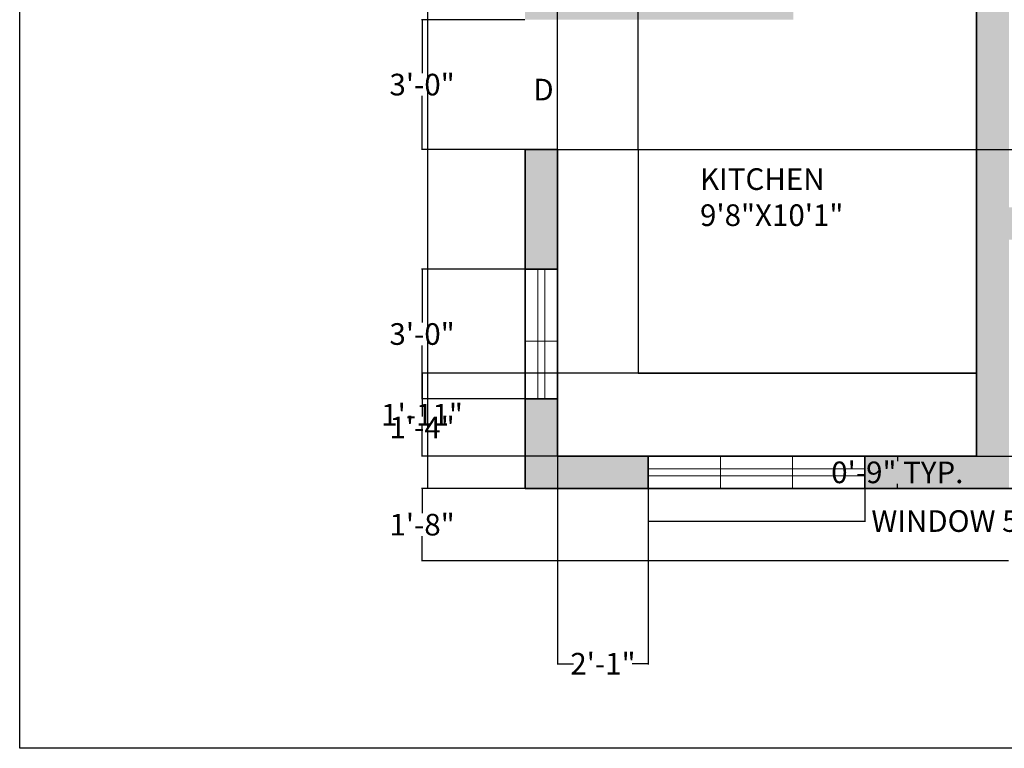
# Model space of a CAD drawing. Units: inches. Extents: x 2552 to 3196, y 4736 to 5443.
# Tile 1 of 8: x 2552 to 2824, y 4736 to 4938. Entities that reach past the tile are written whole.
import ezdxf

# ---------------------------------------------------------------- set-up
doc = ezdxf.new("R2010")
doc.units = ezdxf.units.IN
doc.header["$MEASUREMENT"] = 0
for name, color, linetype, lineweight in [('A-ANNO-DIMS', 2, 'Continuous', 18), ('A-ANNO-TTLB', 7, 'Continuous', 25), ('A-AREA-IDEN', 7, 'Continuous', 18), ('A-DOOR-IDEN', 7, 'Continuous', 18), ('A-FLOR-CASE', 8, 'Continuous', 25), ('A-GLAZ', 4, 'Continuous', 18), ('A-WALL', 7, 'Continuous', 35)]:
    doc.layers.add(name, color=color, linetype=linetype, lineweight=lineweight)
doc.layers.add('A-WALL-PATT', color=30, linetype='Continuous', lineweight=13, true_color=0xf8991e)
doc.styles.get("Standard").update_dxf_attribs({"font": 'arial.ttf'})
doc.dimstyles.get("Standard").update_dxf_attribs({"dimtxt": 6, "dimasz": 0.18, "dimexe": 0.18, "dimexo": 0.0625, "dimgap": 0.09, "dimtad": 0, "dimtih": 1, "dimtoh": 1, "dimdec": 1, "dimzin": 0, "dimdsep": 46, "dimlunit": 3, "dimtxsty": 'Standard', "dimcen": 0.09, "dimadec": 0, "dimazin": 0, "dimtfac": 1, "dimtdec": 1, "dimtofl": 0, "dimtmove": 0, "dimatfit": 3, "dimfxl": 1, "dimtolj": 1, "dimtzin": 0, "dimarcsym": 0})

# ---------------------------------------------------------------- blocks, each defined once
blk = doc.blocks.new('*D1')
at = {"layer": 'A-ANNO-DIMS', "color": 0, "lineweight": -2, "transparency": 16777216}
for p, q in [((2691.59, 5291.32), (2664.57, 5291.32)), ((2664.75, 5291.14), (2664.75, 5052.97)), ((2664.75, 4808.5), (2664.75, 5046.66)), ((2691.59, 4808.32), (2664.57, 4808.32))]:
    blk.add_line(p, q, dxfattribs=at)
at = {"layer": 'A-ANNO-DIMS', "color": 0, "transparency": 16777216}
for points in [[(2664.72, 5291.14), (2664.78, 5291.14), (2664.75, 5291.32)], [(2664.72, 4808.5), (2664.78, 4808.5), (2664.75, 4808.32)]]:
    blk.add_solid(points, dxfattribs=at)
at = {"layer": 'Defpoints', "color": 0, "transparency": 16777216}
for p in [(2691.66, 5291.32), (2664.75, 4808.32), (2691.66, 4808.32)]:
    blk.add_point(p, dxfattribs=at)
at = {"layer": 'A-ANNO-DIMS', "color": 0, "transparency": 16777216, "insert": (2664.75, 5049.82), "char_height": 6, "attachment_point": 5}
blk.add_mtext('\\A1;40\'-3.0"', dxfattribs=at)
blk = doc.blocks.new('WIN-60IN-THREE-LIGHT')
for p, q in [((60, 9), (0, 9)), ((20, 9), (20, 0)), ((40, 0), (40, 9)), ((60, 5.5), (0, 5.5)), ((0, 3.5), (60, 3.5)), ((0, 0), (60, 0))]:
    blk.add_line(p, q)
blk = doc.blocks.new('*D9')
at = {"layer": 'A-ANNO-DIMS', "color": 0, "lineweight": -2, "transparency": 16777216}
for p, q in [((2725.76, 4808.26), (2725.76, 4799.14)), ((2785.76, 4808.26), (2785.76, 4799.14)), ((2725.94, 4799.32), (2785.58, 4799.32)), ((2785.76, 4799.32), (2785.94, 4799.32))]:
    blk.add_line(p, q, dxfattribs=at)
at = {"layer": 'A-ANNO-DIMS', "color": 0, "transparency": 16777216}
for points in [[(2725.94, 4799.35), (2725.94, 4799.29), (2725.76, 4799.32)], [(2785.58, 4799.35), (2785.58, 4799.29), (2785.76, 4799.32)]]:
    blk.add_solid(points, dxfattribs=at)
at = {"layer": 'Defpoints', "color": 0, "transparency": 16777216}
for p in [(2725.76, 4808.32), (2785.76, 4808.32), (2785.76, 4799.32)]:
    blk.add_point(p, dxfattribs=at)
at = {"layer": 'A-ANNO-DIMS', "color": 0, "transparency": 16777216, "insert": (2823.99, 4799.32), "char_height": 6, "attachment_point": 5}
blk.add_mtext('\\A1;WINDOW 5\'-0" TYP.', dxfattribs=at)
blk = doc.blocks.new('*D10')
at = {"layer": 'A-ANNO-DIMS', "color": 0, "lineweight": -2, "transparency": 16777216}
for p, q in [((2785.82, 4817.32), (2794.94, 4817.32)), ((2794.76, 4817.14), (2794.76, 4815.97)), ((2794.76, 4808.5), (2794.76, 4809.66)), ((2785.82, 4808.32), (2794.94, 4808.32))]:
    blk.add_line(p, q, dxfattribs=at)
at = {"layer": 'A-ANNO-DIMS', "color": 0, "transparency": 16777216}
for points in [[(2794.73, 4817.14), (2794.79, 4817.14), (2794.76, 4817.32)], [(2794.73, 4808.5), (2794.79, 4808.5), (2794.76, 4808.32)]]:
    blk.add_solid(points, dxfattribs=at)
at = {"layer": 'Defpoints', "color": 0, "transparency": 16777216}
for p in [(2785.76, 4817.32), (2794.76, 4817.32), (2785.76, 4808.32)]:
    blk.add_point(p, dxfattribs=at)
at = {"layer": 'A-ANNO-DIMS', "color": 0, "transparency": 16777216, "insert": (2794.76, 4812.82), "char_height": 6, "attachment_point": 5}
blk.add_mtext('\\A1;0\'-9" TYP.', dxfattribs=at)
blk = doc.blocks.new('*D23')
at = {"layer": 'A-ANNO-DIMS', "color": 0, "lineweight": -2, "transparency": 16777216}
for p, q in [((2825.59, 4808.32), (2662.93, 4808.32)), ((2663.11, 4808.14), (2663.11, 4801.47)), ((2663.11, 4788.5), (2663.11, 4795.16)), ((2825.59, 4788.32), (2662.93, 4788.32))]:
    blk.add_line(p, q, dxfattribs=at)
at = {"layer": 'A-ANNO-DIMS', "color": 0, "transparency": 16777216}
for points in [[(2663.08, 4808.14), (2663.14, 4808.14), (2663.11, 4808.32)], [(2663.08, 4788.5), (2663.14, 4788.5), (2663.11, 4788.32)]]:
    blk.add_solid(points, dxfattribs=at)
at = {"layer": 'Defpoints', "color": 0, "transparency": 16777216}
for p in [(2663.11, 4808.32), (2825.66, 4808.32), (2825.66, 4788.32)]:
    blk.add_point(p, dxfattribs=at)
at = {"layer": 'A-ANNO-DIMS', "color": 0, "transparency": 16777216, "insert": (2663.11, 4798.32), "char_height": 6, "attachment_point": 5}
blk.add_mtext('\\A1;1\'-8"', dxfattribs=at)
blk = doc.blocks.new('*D28')
at = {"layer": 'A-ANNO-DIMS', "color": 0, "lineweight": -2, "transparency": 16777216}
for p, q in [((2691.59, 4869.17), (2662.93, 4869.17)), ((2663.11, 4868.99), (2663.11, 4854.33)), ((2663.11, 4833.35), (2663.11, 4848.01)), ((2691.59, 4833.17), (2662.93, 4833.17))]:
    blk.add_line(p, q, dxfattribs=at)
at = {"layer": 'A-ANNO-DIMS', "color": 0, "transparency": 16777216}
for points in [[(2663.08, 4868.99), (2663.14, 4868.99), (2663.11, 4869.17)], [(2663.08, 4833.35), (2663.14, 4833.35), (2663.11, 4833.17)]]:
    blk.add_solid(points, dxfattribs=at)
at = {"layer": 'Defpoints', "color": 0, "transparency": 16777216}
for p in [(2663.11, 4869.17), (2691.66, 4869.17), (2691.66, 4833.17)]:
    blk.add_point(p, dxfattribs=at)
at = {"layer": 'A-ANNO-DIMS', "color": 0, "transparency": 16777216, "insert": (2663.11, 4851.17), "char_height": 6, "attachment_point": 5}
blk.add_mtext('\\A1;3\'-0"', dxfattribs=at)
blk = doc.blocks.new('*D37')
at = {"layer": 'A-ANNO-DIMS', "color": 0, "lineweight": -2, "transparency": 16777216}
for p, q in [((2700.66, 4902.38), (2700.66, 5320.05)), ((2700.84, 5319.87), (2722.83, 5319.87)), ((2723.01, 4902.38), (2723.01, 5320.05)), ((2723.01, 5319.87), (2723.19, 5319.87))]:
    blk.add_line(p, q, dxfattribs=at)
at = {"layer": 'A-ANNO-DIMS', "color": 0, "transparency": 16777216}
for points in [[(2700.84, 5319.9), (2700.84, 5319.84), (2700.66, 5319.87)], [(2722.83, 5319.9), (2722.83, 5319.84), (2723.01, 5319.87)]]:
    blk.add_solid(points, dxfattribs=at)
at = {"layer": 'Defpoints', "color": 0, "transparency": 16777216}
for p in [(2723.01, 5319.87), (2700.66, 4902.32), (2723.01, 4902.32)]:
    blk.add_point(p, dxfattribs=at)
at = {"layer": 'A-ANNO-DIMS', "color": 0, "transparency": 16777216, "insert": (2740.29, 5319.87), "char_height": 6, "attachment_point": 5}
blk.add_mtext('\\A1;1\'-10 1/2"', dxfattribs=at)
blk = doc.blocks.new('*D38')
at = {"layer": 'A-ANNO-DIMS', "color": 0, "lineweight": -2, "transparency": 16777216}
for p, q in [((2816.59, 4840.31), (2662.93, 4840.31)), ((2663.11, 4840.13), (2663.11, 4831.91)), ((2663.11, 4817.5), (2663.11, 4825.71)), ((2816.59, 4817.32), (2662.93, 4817.32))]:
    blk.add_line(p, q, dxfattribs=at)
at = {"layer": 'A-ANNO-DIMS', "color": 0, "transparency": 16777216}
for points in [[(2663.08, 4840.13), (2663.14, 4840.13), (2663.11, 4840.31)], [(2663.08, 4817.5), (2663.14, 4817.5), (2663.11, 4817.32)]]:
    blk.add_solid(points, dxfattribs=at)
at = {"layer": 'Defpoints', "color": 0, "transparency": 16777216}
for p in [(2663.11, 4840.31), (2816.66, 4840.31), (2816.66, 4817.32)]:
    blk.add_point(p, dxfattribs=at)
at = {"layer": 'A-ANNO-DIMS', "color": 0, "transparency": 16777216, "insert": (2663.11, 4828.81), "char_height": 6, "attachment_point": 5}
blk.add_mtext('\\A1;1\'-11"', dxfattribs=at)
blk = doc.blocks.new('*D39')
at = {"layer": 'A-ANNO-DIMS', "color": 0, "lineweight": -2, "transparency": 16777216}
for p, q in [((2700.72, 4902.32), (3083.39, 4902.32)), ((3083.21, 4902.14), (3083.21, 4862.92)), ((3083.21, 4817.5), (3083.21, 4856.72)), ((2700.72, 4817.32), (3083.39, 4817.32))]:
    blk.add_line(p, q, dxfattribs=at)
at = {"layer": 'A-ANNO-DIMS', "color": 0, "transparency": 16777216}
for points in [[(3083.18, 4902.14), (3083.24, 4902.14), (3083.21, 4902.32)], [(3083.18, 4817.5), (3083.24, 4817.5), (3083.21, 4817.32)]]:
    blk.add_solid(points, dxfattribs=at)
at = {"layer": 'Defpoints', "color": 0, "transparency": 16777216}
for p in [(2700.66, 4902.32), (3083.21, 4902.32), (2700.66, 4817.32)]:
    blk.add_point(p, dxfattribs=at)
at = {"layer": 'A-ANNO-DIMS', "color": 0, "transparency": 16777216, "insert": (3083.21, 4859.82), "char_height": 6, "attachment_point": 5}
blk.add_mtext('\\A1;7\'-1"', dxfattribs=at)
blk = doc.blocks.new('*D41')
at = {"layer": 'A-ANNO-DIMS', "color": 0, "lineweight": -2, "transparency": 16777216}
for p, q in [((2691.59, 4938.32), (2662.93, 4938.32)), ((2663.11, 4938.14), (2663.11, 4923.47)), ((2663.11, 4902.5), (2663.11, 4917.16)), ((2691.59, 4902.32), (2662.93, 4902.32))]:
    blk.add_line(p, q, dxfattribs=at)
at = {"layer": 'A-ANNO-DIMS', "color": 0, "transparency": 16777216}
for points in [[(2663.08, 4938.14), (2663.14, 4938.14), (2663.11, 4938.32)], [(2663.08, 4902.5), (2663.14, 4902.5), (2663.11, 4902.32)]]:
    blk.add_solid(points, dxfattribs=at)
at = {"layer": 'Defpoints', "color": 0, "transparency": 16777216}
for p in [(2663.11, 4938.32), (2691.66, 4938.32), (2691.66, 4902.32)]:
    blk.add_point(p, dxfattribs=at)
at = {"layer": 'A-ANNO-DIMS', "color": 0, "transparency": 16777216, "insert": (2663.11, 4920.32), "char_height": 6, "attachment_point": 5}
blk.add_mtext('\\A1;3\'-0"', dxfattribs=at)
blk = doc.blocks.new('*D42')
at = {"layer": 'A-ANNO-DIMS', "color": 0, "lineweight": -2, "transparency": 16777216}
for p, q in [((2700.59, 4833.17), (2662.93, 4833.17)), ((2663.11, 4832.99), (2663.11, 4828.35)), ((2663.11, 4817.5), (2663.11, 4822.14)), ((2700.59, 4817.32), (2662.93, 4817.32))]:
    blk.add_line(p, q, dxfattribs=at)
at = {"layer": 'A-ANNO-DIMS', "color": 0, "transparency": 16777216}
for points in [[(2663.08, 4832.99), (2663.14, 4832.99), (2663.11, 4833.17)], [(2663.08, 4817.5), (2663.14, 4817.5), (2663.11, 4817.32)]]:
    blk.add_solid(points, dxfattribs=at)
at = {"layer": 'Defpoints', "color": 0, "transparency": 16777216}
for p in [(2663.11, 4833.17), (2700.66, 4833.17), (2700.66, 4817.32)]:
    blk.add_point(p, dxfattribs=at)
at = {"layer": 'A-ANNO-DIMS', "color": 0, "transparency": 16777216, "insert": (2663.11, 4825.24), "char_height": 6, "attachment_point": 5}
blk.add_mtext('\\A1;1\'-4"', dxfattribs=at)
blk = doc.blocks.new('*D43')
at = {"layer": 'A-ANNO-DIMS', "color": 0, "lineweight": -2, "transparency": 16777216}
for p, q in [((2700.66, 4817.26), (2700.66, 4759.59)), ((2725.76, 4817.26), (2725.76, 4759.59)), ((2700.84, 4759.77), (2705.09, 4759.77)), ((2725.58, 4759.77), (2721.32, 4759.77))]:
    blk.add_line(p, q, dxfattribs=at)
at = {"layer": 'A-ANNO-DIMS', "color": 0, "transparency": 16777216}
for points in [[(2700.84, 4759.8), (2700.84, 4759.74), (2700.66, 4759.77)], [(2725.58, 4759.8), (2725.58, 4759.74), (2725.76, 4759.77)]]:
    blk.add_solid(points, dxfattribs=at)
at = {"layer": 'Defpoints', "color": 0, "transparency": 16777216}
for p in [(2700.66, 4817.32), (2725.76, 4817.32), (2725.76, 4759.77)]:
    blk.add_point(p, dxfattribs=at)
at = {"layer": 'A-ANNO-DIMS', "color": 0, "transparency": 16777216, "insert": (2713.21, 4759.77), "char_height": 6, "attachment_point": 5}
blk.add_mtext('\\A1;2\'-1"', dxfattribs=at)

msp = doc.modelspace()

# ---------------------------------------------------------------- hatches: boundary and pattern name
at = {"layer": 'A-WALL-PATT'}
h = msp.add_hatch(color=256, dxfattribs=at)
h.dxf.hatch_style = 1
h.paths.add_polyline_path([(2700.66, 5282.32), (2732.91, 5282.32), (2732.91, 5291.32), (2691.66, 5291.32), (2691.66, 5248.4), (2700.66, 5248.4)])
h.paths.add_polyline_path([(2865.22, 5291.32), (2792.91, 5291.32), (2792.91, 5282.32), (2839.66, 5282.32), (2839.66, 5136.32), (2848.66, 5136.32), (2848.66, 5182.32), (2913.66, 5182.32), (2913.66, 5246.32), (2904.66, 5246.32), (2904.66, 5191.32), (2848.66, 5191.32), (2848.66, 5282.32), (2865.22, 5282.32)])
h.paths.add_polyline_path([(2946.08, 5291.32), (2889.22, 5291.32), (2889.22, 5282.32), (2946.08, 5282.32)])
h.paths.add_polyline_path([(3054.66, 5291.32), (3006.08, 5291.32), (3006.08, 5282.32), (3045.66, 5282.32), (3045.66, 5249.18), (3054.66, 5249.18)])
h.paths.add_polyline_path([(3054.66, 5189.18), (3045.66, 5189.18), (3045.66, 5145.32), (2904.66, 5145.32), (2904.66, 5136.32), (3045.66, 5136.32), (3045.66, 5103.54), (3054.66, 5103.54)])
h.paths.add_polyline_path([(3054.66, 5043.54), (3045.66, 5043.54), (3045.66, 5012.32), (2913.66, 5012.32), (2913.66, 5100.32), (2904.66, 5100.32), (2904.66, 5003.32), (3045.66, 5003.32), (3045.66, 4980.34), (3054.66, 4980.34)])
h.paths.add_polyline_path([(3054.66, 4920.34), (3045.66, 4920.34), (3045.66, 4886.32), (3029.6, 4886.32), (3029.6, 4877.32), (3045.66, 4877.32), (3045.66, 4817.32), (3041.59, 4817.32), (3041.59, 4808.32), (3054.66, 4808.32)])
h.paths.add_polyline_path([(2996.66, 4877.32), (3013.11, 4877.32), (3013.11, 4886.32), (2987.66, 4886.32), (2987.66, 4808.32), (2999.73, 4808.32), (2999.73, 4817.32), (2996.66, 4817.32)])
h.paths.add_polyline_path([(2825.66, 4877.32), (2853.9, 4877.32), (2853.9, 4886.32), (2825.66, 4886.32), (2825.66, 5000.12), (2816.66, 5000.12), (2816.66, 4817.32), (2785.76, 4817.32), (2785.76, 4808.32), (2825.66, 4808.32)])
h.paths.add_polyline_path([(2951.66, 4886.32), (2913.9, 4886.32), (2913.9, 4877.32), (2951.66, 4877.32)])
h.paths.add_polyline_path([(2725.76, 4817.32), (2700.66, 4817.32), (2700.66, 4833.17), (2691.66, 4833.17), (2691.66, 4808.32), (2725.76, 4808.32)])
h.paths.add_polyline_path([(2700.66, 4902.32), (2691.66, 4902.32), (2691.66, 4869.17), (2700.66, 4869.17)])
h.paths.add_polyline_path([(2765.91, 4947.32), (2700.66, 4947.32), (2700.66, 4977.71), (2691.66, 4977.71), (2691.66, 4938.32), (2765.91, 4938.32)])
h.paths.add_polyline_path([(2825.66, 5077.32), (2773.66, 5077.32), (2773.66, 5112.32), (2764.66, 5112.32), (2764.66, 5077.32), (2700.66, 5077.32), (2700.66, 5102.51), (2691.66, 5102.51), (2691.66, 5037.71), (2700.66, 5037.71), (2700.66, 5068.32), (2816.66, 5068.32), (2816.66, 5036.12), (2825.66, 5036.12)])
h.paths.add_polyline_path([(2803.66, 5145.32), (2700.66, 5145.32), (2700.66, 5188.4), (2691.66, 5188.4), (2691.66, 5126.51), (2700.66, 5126.51), (2700.66, 5136.32), (2803.66, 5136.32)])

# ---------------------------------------------------------------- linework, layer by layer
at = {"layer": 'A-ANNO-TTLB'}
msp.add_lwpolyline([(2551.65, 5442.6), (3195.75, 5442.6), (3195.75, 4736.32), (2551.65, 4736.32)], close=True, dxfattribs=at)
at = {"layer": 'A-FLOR-CASE'}
for p, q in [((2700.66, 4902.32), (2723.01, 4902.32)), ((2723.01, 4902.32), (2723.01, 4840.31)), ((2723.01, 4840.31), (2816.66, 4840.31))]:
    msp.add_line(p, q, dxfattribs=at)
at = {"layer": 'A-GLAZ'}
for p, q in [((2691.66, 4869.17), (2691.66, 4869.17)), ((2691.66, 4869.17), (2691.66, 4833.17)), ((2695.16, 4869.17), (2695.16, 4833.17)), ((2697.16, 4833.17), (2697.16, 4869.17)), ((2700.66, 4833.17), (2700.66, 4869.17)), ((2700.66, 4849.17), (2691.66, 4849.17))]:
    msp.add_line(p, q, dxfattribs=at)
at = {"layer": 'A-WALL'}
for p, q in [((2816.66, 5000.12), (2816.66, 4817.32)), ((2691.66, 4902.32), (2700.66, 4902.32)), ((2691.66, 4902.32), (2691.66, 4808.32)), ((2700.66, 4902.32), (2700.66, 4817.32)), ((2700.66, 4869.17), (2691.66, 4869.17)), ((2691.66, 4833.17), (2700.66, 4833.17)), ((2700.66, 4817.32), (2816.66, 4817.32)), ((2725.76, 4817.32), (2725.76, 4808.32)), ((2785.76, 4808.32), (2785.76, 4817.32)), ((2691.66, 4808.32), (3054.66, 4808.32))]:
    msp.add_line(p, q, dxfattribs=at)

# ---------------------------------------------------------------- block references
at = {"layer": 'A-GLAZ'}
msp.add_blockref('WIN-60IN-THREE-LIGHT', (2725.76, 4808.32), dxfattribs=at)

# ---------------------------------------------------------------- texts
at = {"layer": 'A-AREA-IDEN', "insert": (2740.1, 4897.12), "char_height": 6, "attachment_point": 1}
msp.add_mtext_dynamic_manual_height_columns('KITCHEN\\P9\'8"X10\'1"', width=66.0396, gutter_width=1, heights=[0], dxfattribs=at)
at = {"layer": 'A-DOOR-IDEN', "insert": (2693.93, 4921.93), "char_height": 6, "attachment_point": 1}
msp.add_mtext_dynamic_manual_height_columns('D', width=10.2167, gutter_width=1, heights=[0], dxfattribs=at)

# ---------------------------------------------------------------- dimensions: what is measured, and where the dimension line sits
at = {"layer": 'A-ANNO-DIMS'}
for base, p1, p2, picture, middle in [((2723.00559, 5319.86809), (2700.65555, 4902.31809), (2723.00559, 4902.31809), '*D37', (2740.28923, 5319.86809)), ((2725.76, 4759.77), (2700.66, 4817.32), (2725.76, 4817.32), '*D43', (2713.21, 4759.77))]:
    dim = msp.add_linear_dim(base=base, p1=p1, p2=p2, dimstyle='Standard', override={"dimdec": 1, "dimlfac": 1, "dimrnd": 0, "dimzin": 1, "dimdsep": 46, "dimlunit": 4, "dimfrac": 2}, dxfattribs=at)
    dim.commit()
    dim.dimension.update_dxf_attribs({"geometry": picture, "text_midpoint": middle})
for base, p1, p2, override, picture, middle in [((2664.75, 4808.32), (2691.66, 5291.32), (2691.66, 4808.32), {"dimclrd": 0, "dimclre": 0, "dimclrt": 0}, '*D1', (2664.75, 5049.82)), ((2663.11, 4938.32), (2691.66, 4902.32), (2691.66, 4938.32), {"dimdec": 1, "dimlfac": 1, "dimrnd": 0, "dimzin": 1, "dimdsep": 46, "dimlunit": 4, "dimfrac": 2}, '*D41', (2663.11, 4920.32)), ((3083.21, 4902.32), (2700.66, 4817.32), (2700.66, 4902.32), {"dimdec": 1, "dimlfac": 1, "dimrnd": 0, "dimzin": 1, "dimdsep": 46, "dimlunit": 4, "dimfrac": 2}, '*D39', (3083.21, 4859.82)), ((2663.11, 4869.17), (2691.66, 4833.17), (2691.66, 4869.17), {"dimdec": 1, "dimlfac": 1, "dimrnd": 0, "dimzin": 1, "dimdsep": 46, "dimlunit": 4, "dimfrac": 2}, '*D28', (2663.11, 4851.17)), ((2663.11, 4840.31), (2816.66, 4817.32), (2816.66, 4840.31), {"dimdec": 1, "dimlfac": 1, "dimrnd": 0, "dimzin": 1, "dimdsep": 46, "dimlunit": 4, "dimfrac": 2}, '*D38', (2663.11, 4828.81)), ((2663.1056, 4833.1702), (2700.6556, 4817.3181), (2700.6556, 4833.1702), {"dimdec": 1, "dimlfac": 1, "dimrnd": 0, "dimzin": 1, "dimdsep": 46, "dimlunit": 4, "dimfrac": 2}, '*D42', (2663.1056, 4825.2441)), ((2663.11, 4808.32), (2825.66, 4788.32), (2825.66, 4808.32), {"dimdec": 1, "dimlfac": 1, "dimrnd": 0, "dimzin": 1, "dimdsep": 46, "dimlunit": 4, "dimfrac": 2}, '*D23', (2663.11, 4798.32))]:
    dim = msp.add_linear_dim(base=base, p1=p1, p2=p2, angle=90, dimstyle='Standard', override=override, dxfattribs=at)
    dim.commit()
    dim.dimension.update_dxf_attribs({"geometry": picture, "text_midpoint": middle})
dim = msp.add_linear_dim(base=(2794.76, 4817.32), p1=(2785.76, 4808.32), p2=(2785.76, 4817.32), angle=90, text='<> TYP.', dimstyle='Standard', override={"dimdec": 1, "dimlfac": 1, "dimrnd": 0, "dimzin": 1, "dimdsep": 46, "dimlunit": 4, "dimfrac": 2}, dxfattribs=at)
dim.commit()
dim.dimension.update_dxf_attribs({"geometry": '*D10', "text_midpoint": (2794.76, 4812.82)})
dim = msp.add_linear_dim(base=(2785.76, 4799.32), p1=(2725.76, 4808.32), p2=(2785.76, 4808.32), text='WINDOW <> TYP.', dimstyle='Standard', override={"dimdec": 1, "dimlfac": 1, "dimrnd": 0, "dimzin": 1, "dimdsep": 46, "dimlunit": 4, "dimfrac": 2}, dxfattribs=at)
dim.commit()
dim.dimension.update_dxf_attribs({"geometry": '*D9', "text_midpoint": (2823.99, 4799.32)})

doc.saveas('drawing.dxf')
